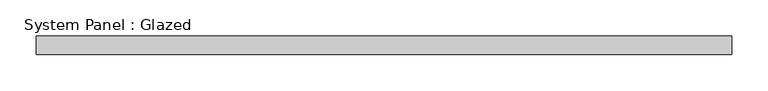
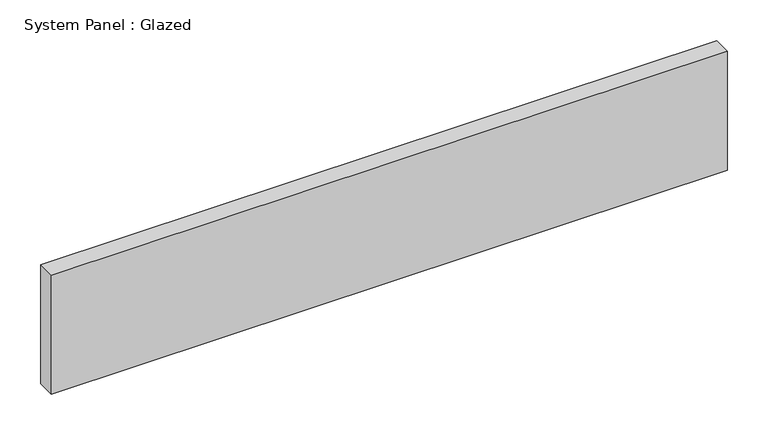
"""IFC4 building model written with IfcOpenShell, lengths in millimetres: plate geometry, System Panel : Glazed."""

from ifc_helpers import new_model, si_unit, origin, origin_with_axes, place, context, project, spatial, polyline, outline, extrude, source, transform, mapped, element, save


def system_panel_glazed_eb071a3d(model_context):
    return source(origin(), model_context, "Body", "SweptSolid", [
        extrude(outline(polyline([(477.3083334, 19.05), (-477.3083334, 19.05), (-477.3083334, 44.45), (477.3083334, 44.45), (477.3083334, 19.05)])), origin_with_axes(), (0.0, 0.0, 1.0), 177.8),
    ])


if __name__ == "__main__":
    model = new_model("IFC4")
    model_context = context("Model", 3, world=origin())
    ifc_project = project(units=[si_unit("LENGTHUNIT", "METRE", prefix="MILLI")], contexts=[model_context])
    site = spatial("IfcSite", under=ifc_project)
    building = spatial("IfcBuilding", under=site)
    placement = place(None, origin())
    system_panel_glazed_shape = system_panel_glazed_eb071a3d(model_context)
    element("IfcPlate", 1, ObjectType="System Panel : Glazed", at=placement, inside=building, context=model_context, shape_type="MappedRepresentation", body=[
        mapped(system_panel_glazed_shape, transform((0.0, 0.0, 0.0), x_axis=(1.0, 0.0, 0.0), y_axis=(0.0, 1.0, 0.0), z_axis=(0.0, 0.0, 1.0))),
    ])
    save(model, "model.ifc")

# Revit data of these elements
# Type "System Panel : Glazed"
#   Construction Type Id = "GSP4R"
#   Analytic Construction = "1/8 in Pilkington single glazing"
#   Visual Light Transmittance = 0.9
#   Solar Heat Gain Coefficient = 0.86
#   Heat Transfer Coefficient (U) = 1.18115 BTU/(h·ft²·°F)
#   Define Thermal Properties by = 1
# Element 1 (IfcPlate, "System Panel : Glazed")
#   Materials on its faces: "Glass"
# Materials
#   "Glass": class "Glass", colour RGB 0 128 192, transparency 0.75, Description = "Soda Lime Glass", Cost = 0
